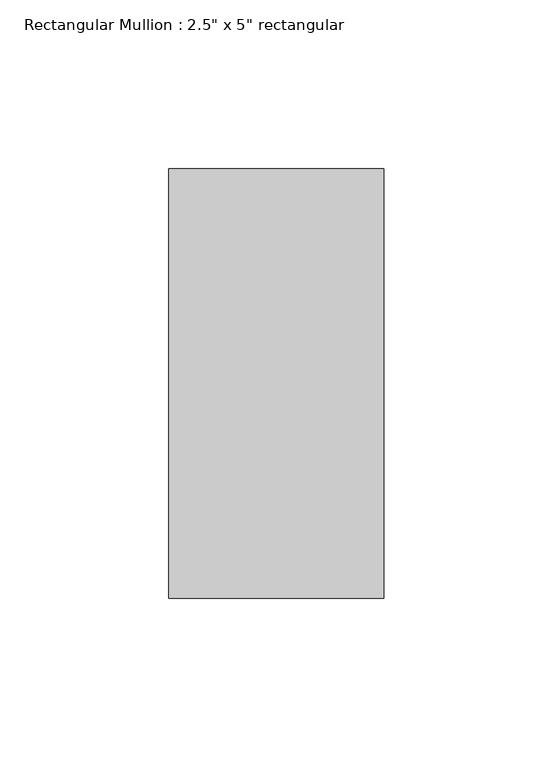
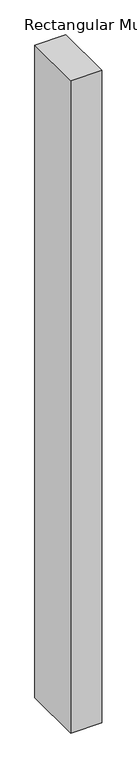
"""IFC4 building model written with IfcOpenShell, lengths in millimetres: member geometry."""

from ifc_helpers import new_model, si_unit, frame, origin, place, context, project, spatial, polyline, outline, extrude, source, transform, mapped, element, save


def member_4de4f528(model_context):
    return source(origin(), model_context, "Body", "SweptSolid", [
        extrude(outline(polyline([(0.0, 63.5), (0.0, -63.5), (-63.5, -63.5), (-63.5, 63.5), (0.0, 63.5)])), frame((0.0, 0.0, -1415.2315053), z_axis=(0.0, 0.0, 1.0), x_axis=(1.0, 0.0, 0.0)), (0.0, 0.0, 1.0), 1415.2315053),
    ])


if __name__ == "__main__":
    model = new_model("IFC4")
    model_context = context("Model", 3, world=origin())
    ifc_project = project(units=[si_unit("LENGTHUNIT", "METRE", prefix="MILLI")], contexts=[model_context])
    site = spatial("IfcSite", under=ifc_project)
    building = spatial("IfcBuilding", under=site)
    placement = place(None, origin())
    member_shape = member_4de4f528(model_context)
    element("IfcMember", 1, ObjectType="Rectangular Mullion : 2.5\" x 5\" rectangular", at=placement, inside=building, context=model_context, shape_type="MappedRepresentation", body=[
        mapped(member_shape, transform((0.0, 0.0, 0.0), x_axis=(1.0, 0.0, 0.0), y_axis=(0.0, 1.0, 0.0), z_axis=(0.0, 0.0, 1.0))),
    ])
    save(model, "model.ifc")

# Revit data of these elements
# Type "Rectangular Mullion : 2.5\" x 5\" rectangular"
#   built-in parameter 1007304 = 0.416667 (stored number, unit not read)
#   built-in parameter 1007301 = 0.104167 (stored number, unit not read)
#   built-in parameter 1007300 = 0.104167 (stored number, unit not read)
# Element 1 (IfcMember, "Rectangular Mullion : 2.5\" x 5\" rectangular")
#   Materials on its faces: "mullions"
# Materials
#   "mullions": class "Generic", colour RGB 120 120 120, transparency 0, Cost = 0
